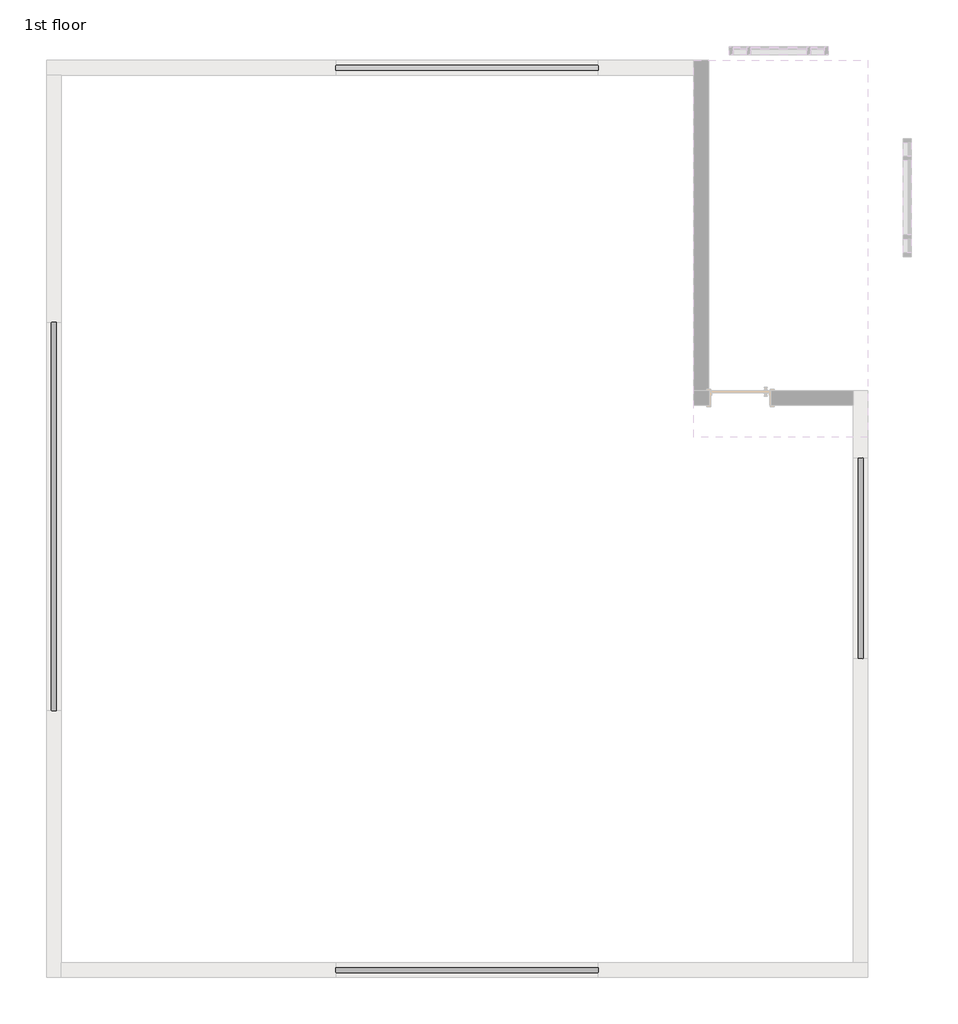
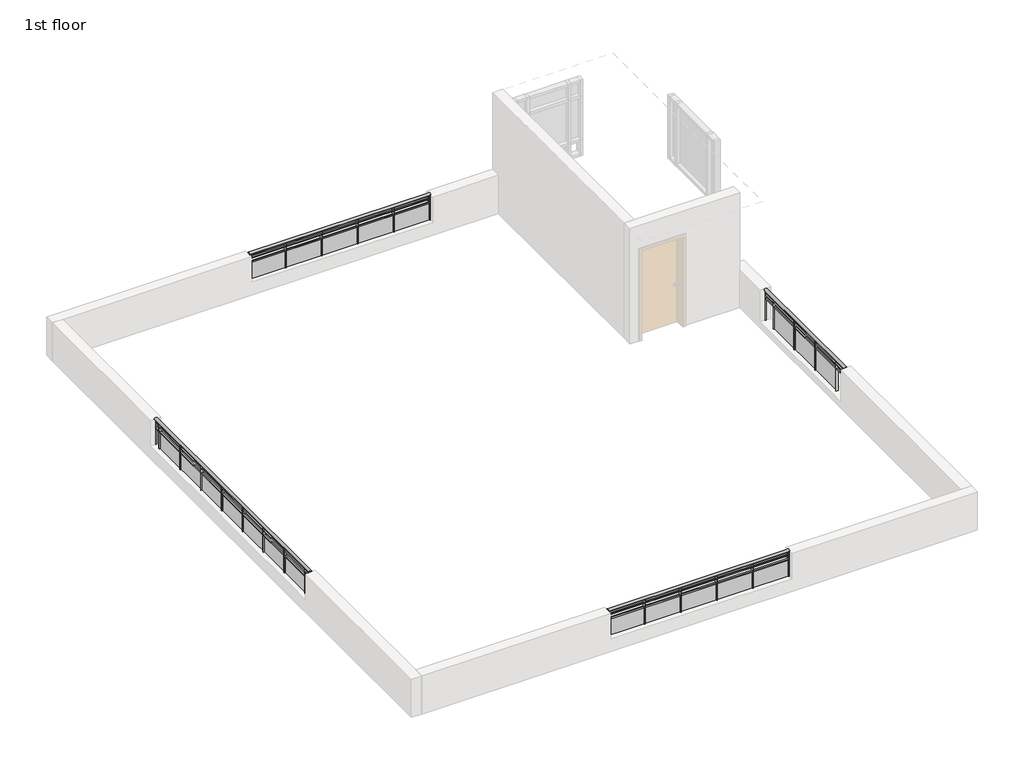
# One storey, part 2 of 2: 4 railings.
"""IFC4 building model written with IfcOpenShell, lengths in millimetres."""

from ifc_helpers import new_model, si_unit, point, frame, origin, place, context, project, spatial, polyline, ellipse_curve, trimmed, outline, extrude, element, save
from ifc_brep_helpers import plane_surface, extruded_surface, advanced_brep

model = new_model("IFC4")

# Units and contexts
model_context = context("Model", 3, world=origin())
ifc_project = project(units=[si_unit("LENGTHUNIT", "METRE", prefix="MILLI")], contexts=[model_context])

# Site, building, storey
site = spatial("IfcSite", under=ifc_project)
building = spatial("IfcBuilding", under=site)
storey = spatial("IfcBuildingStorey", under=building, Name="1st floor", Elevation=3200.4)

# Railings
placement = place(None, origin())
element("IfcRailing", 1, ObjectType="Glass Panel - Bottom Fill", at=placement, inside=storey, context=model_context, shape_type="SolidModel", body=[
    advanced_brep(
    [(186.9722402, 5808.6342801, 4086.225), (110.7722402, 5808.6342801, 4086.225), (186.9722402, 2680.2485536, 4086.225), (110.7722402, 2680.2485536, 4086.225)],
    [
        (0, 1, ellipse_curve(frame((148.8722402, 5808.6342801, 4086.225), z_axis=(0.0, 1.0, 0.0), x_axis=(-1.0, 0.0, 0.0)), 38.1, 28.575)),
        (1, 0, ellipse_curve(frame((148.8722402, 5808.6342801, 4086.225), z_axis=(0.0, 1.0, 0.0), x_axis=(-1.0, 0.0, 0.0)), 38.1, 28.575)),
        (2, 3, ellipse_curve(frame((148.8722402, 2680.2485536, 4086.225), z_axis=(0.0, -1.0, 0.0), x_axis=(-1.0, 0.0, 0.0)), 38.1, 28.575)),
        (3, 2, ellipse_curve(frame((148.8722402, 2680.2485536, 4086.225), z_axis=(0.0, -1.0, 0.0), x_axis=(-1.0, 0.0, 0.0)), 38.1, 28.575)),
        (0, 2),
        (3, 1),
    ],
    [
        plane_surface(frame((148.8722402, 5808.6342801, 4086.225), z_axis=(0.0, 1.0, 0.0), x_axis=(0.0, 0.0, -1.0))),
        plane_surface(frame((148.8722402, 2680.2485536, 4086.225), z_axis=(0.0, -1.0, 0.0), x_axis=(0.0, 0.0, -1.0))),
        extruded_surface(trimmed(ellipse_curve(frame((148.8722402, 2680.2485536, 4086.225), z_axis=(0.0, 1.0, 0.0), x_axis=(-1.0, 0.0, 0.0)), 38.1, 28.575), [point((186.9722402, 2680.2485536, 4086.225))], [point((110.7722402, 2680.2485536, 4086.225))], True, "CARTESIAN"), (0.0, 3128.3857265, 0.0), 3128.3857265),
        extruded_surface(trimmed(ellipse_curve(frame((148.8722402, 2680.2485536, 4086.225), z_axis=(0.0, 1.0, 0.0), x_axis=(-1.0, 0.0, 0.0)), 38.1, 28.575), [point((110.7722402, 2680.2485536, 4086.225))], [point((186.9722402, 2680.2485536, 4086.225))], True, "CARTESIAN"), (0.0, 3128.3857265, 0.0), 3128.3857265),
    ],
    [
        (0, [[1, 2]]),
        (1, [[3, 4]]),
        (2, [[-1, 5, -4, 6]]),
        (3, [[-2, -6, -3, -5]]),
    ],
),
    extrude(outline(polyline([(136.1722402, 5808.6342801), (161.5722402, 5808.6342801), (161.5722402, 2680.2485536), (136.1722402, 2680.2485536), (136.1722402, 5808.6342801)])), frame((0.0, 0.0, 3971.925), z_axis=(0.0, 0.0, 1.0), x_axis=(1.0, 0.0, 0.0)), (0.0, 0.0, 1.0), 25.4),
    extrude(outline(polyline([(136.1722402, 5808.6342801), (161.5722402, 5808.6342801), (161.5722402, 2680.2485536), (136.1722402, 2680.2485536), (136.1722402, 5808.6342801)])), frame((0.0, 0.0, 3870.325), z_axis=(0.0, 0.0, 1.0), x_axis=(1.0, 0.0, 0.0)), (0.0, 0.0, 1.0), 25.4),
    extrude(outline(polyline([(123.4722402, 3031.5914169), (174.2722402, 3031.5914169), (174.2722402, 3018.8914169), (123.4722402, 3018.8914169), (123.4722402, 3031.5914169)])), frame((0.0, 0.0, 3171.825), z_axis=(0.0, 0.0, 1.0), x_axis=(1.0, 0.0, 0.0)), (0.0, 0.0, 1.0), 885.825),
    extrude(outline(polyline([(155.4073972, 3838.0414169), (155.4073972, 3025.2414169), (149.0573972, 3025.2414169), (149.0573972, 3838.0414169), (155.4073972, 3838.0414169)])), frame((0.0, 0.0, 3273.425), z_axis=(0.0, 0.0, 1.0), x_axis=(1.0, 0.0, 0.0)), (0.0, 0.0, 1.0), 596.9),
    extrude(outline(polyline([(123.4722402, 3844.3914169), (174.2722402, 3844.3914169), (174.2722402, 3831.6914169), (123.4722402, 3831.6914169), (123.4722402, 3844.3914169)])), frame((0.0, 0.0, 3171.825), z_axis=(0.0, 0.0, 1.0), x_axis=(1.0, 0.0, 0.0)), (0.0, 0.0, 1.0), 885.825),
    extrude(outline(polyline([(155.4073972, 4650.8414169), (155.4073972, 3838.0414169), (149.0573972, 3838.0414169), (149.0573972, 4650.8414169), (155.4073972, 4650.8414169)])), frame((0.0, 0.0, 3273.425), z_axis=(0.0, 0.0, 1.0), x_axis=(1.0, 0.0, 0.0)), (0.0, 0.0, 1.0), 596.9),
    extrude(outline(polyline([(123.4722402, 4657.1914169), (174.2722402, 4657.1914169), (174.2722402, 4644.4914169), (123.4722402, 4644.4914169), (123.4722402, 4657.1914169)])), frame((0.0, 0.0, 3171.825), z_axis=(0.0, 0.0, 1.0), x_axis=(1.0, 0.0, 0.0)), (0.0, 0.0, 1.0), 885.825),
    extrude(outline(polyline([(155.4073972, 5463.6414169), (155.4073972, 4650.8414169), (149.0573972, 4650.8414169), (149.0573972, 5463.6414169), (155.4073972, 5463.6414169)])), frame((0.0, 0.0, 3273.425), z_axis=(0.0, 0.0, 1.0), x_axis=(1.0, 0.0, 0.0)), (0.0, 0.0, 1.0), 596.9),
    extrude(outline(polyline([(123.4722402, 5469.9914169), (174.2722402, 5469.9914169), (174.2722402, 5457.2914169), (123.4722402, 5457.2914169), (123.4722402, 5469.9914169)])), frame((0.0, 0.0, 3171.825), z_axis=(0.0, 0.0, 1.0), x_axis=(1.0, 0.0, 0.0)), (0.0, 0.0, 1.0), 885.825),
    extrude(outline(polyline([(139.3472402, 2692.9485536), (158.3972402, 2692.9485536), (158.3972402, 2673.8985536), (139.3472402, 2673.8985536), (139.3472402, 2692.9485536)])), frame((0.0, 0.0, 3171.825), z_axis=(0.0, 0.0, 1.0), x_axis=(1.0, 0.0, 0.0)), (0.0, 0.0, 1.0), 885.825),
    extrude(outline(polyline([(139.3472402, 5814.9842801), (158.3972402, 5814.9842801), (158.3972402, 5795.9342801), (139.3472402, 5795.9342801), (139.3472402, 5814.9842801)])), frame((0.0, 0.0, 3171.825), z_axis=(0.0, 0.0, 1.0), x_axis=(1.0, 0.0, 0.0)), (0.0, 0.0, 1.0), 885.825),
])
element("IfcRailing", 2, ObjectType="Glass Panel - Bottom Fill", at=placement, inside=storey, context=model_context, shape_type="SolidModel", body=[
    advanced_brep(
    [(-8005.6015325, -2116.1657199, 4114.8), (-8005.6015325, -2192.3657199, 4114.8), (-3926.753987, -2116.1657199, 4114.8), (-3926.753987, -2192.3657199, 4114.8)],
    [
        (0, 1, ellipse_curve(frame((-8005.6015325, -2154.2657199, 4114.8), z_axis=(-1.0, 0.0, 0.0), x_axis=(0.0, -1.0, 0.0)), 38.1, 28.575)),
        (1, 0, ellipse_curve(frame((-8005.6015325, -2154.2657199, 4114.8), z_axis=(-1.0, 0.0, 0.0), x_axis=(0.0, -1.0, 0.0)), 38.1, 28.575)),
        (2, 3, ellipse_curve(frame((-3926.753987, -2154.2657199, 4114.8), z_axis=(1.0, 0.0, 0.0), x_axis=(0.0, -1.0, 0.0)), 38.1, 28.575)),
        (3, 2, ellipse_curve(frame((-3926.753987, -2154.2657199, 4114.8), z_axis=(1.0, 0.0, 0.0), x_axis=(0.0, -1.0, 0.0)), 38.1, 28.575)),
        (0, 2),
        (3, 1),
    ],
    [
        plane_surface(frame((-8005.6015325, -2154.2657199, 4114.8), z_axis=(-1.0, 0.0, 0.0), x_axis=(0.0, 1.0, 0.0))),
        plane_surface(frame((-3926.753987, -2154.2657199, 4114.8), z_axis=(1.0, 0.0, 0.0), x_axis=(0.0, 1.0, 0.0))),
        extruded_surface(trimmed(ellipse_curve(frame((-3926.753987, -2154.2657199, 4114.8), z_axis=(-1.0, 0.0, 0.0), x_axis=(0.0, -1.0, 0.0)), 38.1, 28.575), [point((-3926.753987, -2116.1657199, 4114.8))], [point((-3926.753987, -2192.3657199, 4114.8))], True, "CARTESIAN"), (-4078.8475455, 0.0, 0.0), 4078.8475455),
        extruded_surface(trimmed(ellipse_curve(frame((-3926.753987, -2154.2657199, 4114.8), z_axis=(-1.0, 0.0, 0.0), x_axis=(0.0, -1.0, 0.0)), 38.1, 28.575), [point((-3926.753987, -2192.3657199, 4114.8))], [point((-3926.753987, -2116.1657199, 4114.8))], True, "CARTESIAN"), (-4078.8475455, 0.0, 0.0), 4078.8475455),
    ],
    [
        (0, [[1, 2]]),
        (1, [[3, 4]]),
        (2, [[-1, 5, -4, 6]]),
        (3, [[-2, -6, -3, -5]]),
    ],
),
    extrude(outline(polyline([(-8005.6015325, -2166.9657199), (-8005.6015325, -2141.5657199), (-3926.753987, -2141.5657199), (-3926.753987, -2166.9657199), (-8005.6015325, -2166.9657199)])), frame((0.0, 0.0, 4000.5), z_axis=(0.0, 0.0, 1.0), x_axis=(1.0, 0.0, 0.0)), (0.0, 0.0, 1.0), 25.4),
    extrude(outline(polyline([(-8005.6015325, -2166.9657199), (-8005.6015325, -2141.5657199), (-3926.753987, -2141.5657199), (-3926.753987, -2166.9657199), (-8005.6015325, -2166.9657199)])), frame((0.0, 0.0, 3898.9), z_axis=(0.0, 0.0, 1.0), x_axis=(1.0, 0.0, 0.0)), (0.0, 0.0, 1.0), 25.4),
    extrude(outline(polyline([(-3940.5277598, -2179.6657199), (-3940.5277598, -2128.8657199), (-3927.8277598, -2128.8657199), (-3927.8277598, -2179.6657199), (-3940.5277598, -2179.6657199)])), frame((0.0, 0.0, 3200.4), z_axis=(0.0, 0.0, 1.0), x_axis=(1.0, 0.0, 0.0)), (0.0, 0.0, 1.0), 885.825),
    extrude(outline(polyline([(-4746.9777598, -2147.7305629), (-3934.1777598, -2147.7305629), (-3934.1777598, -2154.0805629), (-4746.9777598, -2154.0805629), (-4746.9777598, -2147.7305629)])), frame((0.0, 0.0, 3302.0), z_axis=(0.0, 0.0, 1.0), x_axis=(1.0, 0.0, 0.0)), (0.0, 0.0, 1.0), 596.9),
    extrude(outline(polyline([(-4753.3277598, -2179.6657199), (-4753.3277598, -2128.8657199), (-4740.6277598, -2128.8657199), (-4740.6277598, -2179.6657199), (-4753.3277598, -2179.6657199)])), frame((0.0, 0.0, 3200.4), z_axis=(0.0, 0.0, 1.0), x_axis=(1.0, 0.0, 0.0)), (0.0, 0.0, 1.0), 885.825),
    extrude(outline(polyline([(-5559.7777598, -2147.7305629), (-4746.9777598, -2147.7305629), (-4746.9777598, -2154.0805629), (-5559.7777598, -2154.0805629), (-5559.7777598, -2147.7305629)])), frame((0.0, 0.0, 3302.0), z_axis=(0.0, 0.0, 1.0), x_axis=(1.0, 0.0, 0.0)), (0.0, 0.0, 1.0), 596.9),
    extrude(outline(polyline([(-5566.1277598, -2179.6657199), (-5566.1277598, -2128.8657199), (-5553.4277598, -2128.8657199), (-5553.4277598, -2179.6657199), (-5566.1277598, -2179.6657199)])), frame((0.0, 0.0, 3200.4), z_axis=(0.0, 0.0, 1.0), x_axis=(1.0, 0.0, 0.0)), (0.0, 0.0, 1.0), 885.825),
    extrude(outline(polyline([(-6372.5777598, -2147.7305629), (-5559.7777598, -2147.7305629), (-5559.7777598, -2154.0805629), (-6372.5777598, -2154.0805629), (-6372.5777598, -2147.7305629)])), frame((0.0, 0.0, 3302.0), z_axis=(0.0, 0.0, 1.0), x_axis=(1.0, 0.0, 0.0)), (0.0, 0.0, 1.0), 596.9),
    extrude(outline(polyline([(-6378.9277598, -2179.6657199), (-6378.9277598, -2128.8657199), (-6366.2277598, -2128.8657199), (-6366.2277598, -2179.6657199), (-6378.9277598, -2179.6657199)])), frame((0.0, 0.0, 3200.4), z_axis=(0.0, 0.0, 1.0), x_axis=(1.0, 0.0, 0.0)), (0.0, 0.0, 1.0), 885.825),
    extrude(outline(polyline([(-7185.3777598, -2147.7305629), (-6372.5777598, -2147.7305629), (-6372.5777598, -2154.0805629), (-7185.3777598, -2154.0805629), (-7185.3777598, -2147.7305629)])), frame((0.0, 0.0, 3302.0), z_axis=(0.0, 0.0, 1.0), x_axis=(1.0, 0.0, 0.0)), (0.0, 0.0, 1.0), 596.9),
    extrude(outline(polyline([(-7191.7277598, -2179.6657199), (-7191.7277598, -2128.8657199), (-7179.0277598, -2128.8657199), (-7179.0277598, -2179.6657199), (-7191.7277598, -2179.6657199)])), frame((0.0, 0.0, 3200.4), z_axis=(0.0, 0.0, 1.0), x_axis=(1.0, 0.0, 0.0)), (0.0, 0.0, 1.0), 885.825),
    extrude(outline(polyline([(-7998.1777598, -2147.7305629), (-7185.3777598, -2147.7305629), (-7185.3777598, -2154.0805629), (-7998.1777598, -2154.0805629), (-7998.1777598, -2147.7305629)])), frame((0.0, 0.0, 3302.0), z_axis=(0.0, 0.0, 1.0), x_axis=(1.0, 0.0, 0.0)), (0.0, 0.0, 1.0), 596.9),
    extrude(outline(polyline([(-8004.5277598, -2179.6657199), (-8004.5277598, -2128.8657199), (-7991.8277598, -2128.8657199), (-7991.8277598, -2179.6657199), (-8004.5277598, -2179.6657199)])), frame((0.0, 0.0, 3200.4), z_axis=(0.0, 0.0, 1.0), x_axis=(1.0, 0.0, 0.0)), (0.0, 0.0, 1.0), 885.825),
    extrude(outline(polyline([(-3939.453987, -2163.7907199), (-3939.453987, -2144.7407199), (-3920.403987, -2144.7407199), (-3920.403987, -2163.7907199), (-3939.453987, -2163.7907199)])), frame((0.0, 0.0, 3200.4), z_axis=(0.0, 0.0, 1.0), x_axis=(1.0, 0.0, 0.0)), (0.0, 0.0, 1.0), 885.825),
    extrude(outline(polyline([(-8011.9515325, -2163.7907199), (-8011.9515325, -2144.7407199), (-7992.9015325, -2144.7407199), (-7992.9015325, -2163.7907199), (-8011.9515325, -2163.7907199)])), frame((0.0, 0.0, 3200.4), z_axis=(0.0, 0.0, 1.0), x_axis=(1.0, 0.0, 0.0)), (0.0, 0.0, 1.0), 885.825),
])
element("IfcRailing", 3, ObjectType="Glass Panel - Bottom Fill", at=placement, inside=storey, context=model_context, shape_type="SolidModel", body=[
    advanced_brep(
    [(-12347.9277598, 7909.3467978, 4114.8), (-12424.1277598, 7909.3467978, 4114.8), (-12347.9277598, 1879.1217625, 4114.8), (-12424.1277598, 1879.1217625, 4114.8)],
    [
        (0, 1, ellipse_curve(frame((-12386.0277598, 7909.3467978, 4114.8), z_axis=(0.0, 1.0, 0.0), x_axis=(-1.0, 0.0, 0.0)), 38.1, 28.575)),
        (1, 0, ellipse_curve(frame((-12386.0277598, 7909.3467978, 4114.8), z_axis=(0.0, 1.0, 0.0), x_axis=(-1.0, 0.0, 0.0)), 38.1, 28.575)),
        (2, 3, ellipse_curve(frame((-12386.0277598, 1879.1217625, 4114.8), z_axis=(0.0, -1.0, 0.0), x_axis=(-1.0, 0.0, 0.0)), 38.1, 28.575)),
        (3, 2, ellipse_curve(frame((-12386.0277598, 1879.1217625, 4114.8), z_axis=(0.0, -1.0, 0.0), x_axis=(-1.0, 0.0, 0.0)), 38.1, 28.575)),
        (0, 2),
        (3, 1),
    ],
    [
        plane_surface(frame((-12386.0277598, 7909.3467978, 4114.8), z_axis=(0.0, 1.0, 0.0), x_axis=(0.0, 0.0, -1.0))),
        plane_surface(frame((-12386.0277598, 1879.1217625, 4114.8), z_axis=(0.0, -1.0, 0.0), x_axis=(0.0, 0.0, -1.0))),
        extruded_surface(trimmed(ellipse_curve(frame((-12386.0277598, 1879.1217625, 4114.8), z_axis=(0.0, 1.0, 0.0), x_axis=(-1.0, 0.0, 0.0)), 38.1, 28.575), [point((-12347.9277598, 1879.1217625, 4114.8))], [point((-12424.1277598, 1879.1217625, 4114.8))], True, "CARTESIAN"), (0.0, 6030.2250353, 0.0), 6030.2250353),
        extruded_surface(trimmed(ellipse_curve(frame((-12386.0277598, 1879.1217625, 4114.8), z_axis=(0.0, 1.0, 0.0), x_axis=(-1.0, 0.0, 0.0)), 38.1, 28.575), [point((-12424.1277598, 1879.1217625, 4114.8))], [point((-12347.9277598, 1879.1217625, 4114.8))], True, "CARTESIAN"), (0.0, 6030.2250353, 0.0), 6030.2250353),
    ],
    [
        (0, [[1, 2]]),
        (1, [[3, 4]]),
        (2, [[-1, 5, -4, 6]]),
        (3, [[-2, -6, -3, -5]]),
    ],
),
    extrude(outline(polyline([(-12398.7277598, 7909.3467978), (-12373.3277598, 7909.3467978), (-12373.3277598, 1879.1217625), (-12398.7277598, 1879.1217625), (-12398.7277598, 7909.3467978)])), frame((0.0, 0.0, 4000.5), z_axis=(0.0, 0.0, 1.0), x_axis=(1.0, 0.0, 0.0)), (0.0, 0.0, 1.0), 25.4),
    extrude(outline(polyline([(-12398.7277598, 7909.3467978), (-12373.3277598, 7909.3467978), (-12373.3277598, 1879.1217625), (-12398.7277598, 1879.1217625), (-12398.7277598, 7909.3467978)])), frame((0.0, 0.0, 3898.9), z_axis=(0.0, 0.0, 1.0), x_axis=(1.0, 0.0, 0.0)), (0.0, 0.0, 1.0), 25.4),
    extrude(outline(polyline([(-12411.4277598, 2055.7842801), (-12360.6277598, 2055.7842801), (-12360.6277598, 2043.0842801), (-12411.4277598, 2043.0842801), (-12411.4277598, 2055.7842801)])), frame((0.0, 0.0, 3200.4), z_axis=(0.0, 0.0, 1.0), x_axis=(1.0, 0.0, 0.0)), (0.0, 0.0, 1.0), 885.825),
    extrude(outline(polyline([(-12379.4926028, 2862.2342801), (-12379.4926028, 2049.4342801), (-12385.8426028, 2049.4342801), (-12385.8426028, 2862.2342801), (-12379.4926028, 2862.2342801)])), frame((0.0, 0.0, 3302.0), z_axis=(0.0, 0.0, 1.0), x_axis=(1.0, 0.0, 0.0)), (0.0, 0.0, 1.0), 596.9),
    extrude(outline(polyline([(-12411.4277598, 2868.5842801), (-12360.6277598, 2868.5842801), (-12360.6277598, 2855.8842801), (-12411.4277598, 2855.8842801), (-12411.4277598, 2868.5842801)])), frame((0.0, 0.0, 3200.4), z_axis=(0.0, 0.0, 1.0), x_axis=(1.0, 0.0, 0.0)), (0.0, 0.0, 1.0), 885.825),
    extrude(outline(polyline([(-12379.4926028, 3675.0342801), (-12379.4926028, 2862.2342801), (-12385.8426028, 2862.2342801), (-12385.8426028, 3675.0342801), (-12379.4926028, 3675.0342801)])), frame((0.0, 0.0, 3302.0), z_axis=(0.0, 0.0, 1.0), x_axis=(1.0, 0.0, 0.0)), (0.0, 0.0, 1.0), 596.9),
    extrude(outline(polyline([(-12411.4277598, 3681.3842801), (-12360.6277598, 3681.3842801), (-12360.6277598, 3668.6842801), (-12411.4277598, 3668.6842801), (-12411.4277598, 3681.3842801)])), frame((0.0, 0.0, 3200.4), z_axis=(0.0, 0.0, 1.0), x_axis=(1.0, 0.0, 0.0)), (0.0, 0.0, 1.0), 885.825),
    extrude(outline(polyline([(-12379.4926028, 4487.8342801), (-12379.4926028, 3675.0342801), (-12385.8426028, 3675.0342801), (-12385.8426028, 4487.8342801), (-12379.4926028, 4487.8342801)])), frame((0.0, 0.0, 3302.0), z_axis=(0.0, 0.0, 1.0), x_axis=(1.0, 0.0, 0.0)), (0.0, 0.0, 1.0), 596.9),
    extrude(outline(polyline([(-12411.4277598, 4494.1842801), (-12360.6277598, 4494.1842801), (-12360.6277598, 4481.4842801), (-12411.4277598, 4481.4842801), (-12411.4277598, 4494.1842801)])), frame((0.0, 0.0, 3200.4), z_axis=(0.0, 0.0, 1.0), x_axis=(1.0, 0.0, 0.0)), (0.0, 0.0, 1.0), 885.825),
    extrude(outline(polyline([(-12379.4926028, 5300.6342801), (-12379.4926028, 4487.8342801), (-12385.8426028, 4487.8342801), (-12385.8426028, 5300.6342801), (-12379.4926028, 5300.6342801)])), frame((0.0, 0.0, 3302.0), z_axis=(0.0, 0.0, 1.0), x_axis=(1.0, 0.0, 0.0)), (0.0, 0.0, 1.0), 596.9),
    extrude(outline(polyline([(-12411.4277598, 5306.9842801), (-12360.6277598, 5306.9842801), (-12360.6277598, 5294.2842801), (-12411.4277598, 5294.2842801), (-12411.4277598, 5306.9842801)])), frame((0.0, 0.0, 3200.4), z_axis=(0.0, 0.0, 1.0), x_axis=(1.0, 0.0, 0.0)), (0.0, 0.0, 1.0), 885.825),
    extrude(outline(polyline([(-12379.4926028, 6113.4342801), (-12379.4926028, 5300.6342801), (-12385.8426028, 5300.6342801), (-12385.8426028, 6113.4342801), (-12379.4926028, 6113.4342801)])), frame((0.0, 0.0, 3302.0), z_axis=(0.0, 0.0, 1.0), x_axis=(1.0, 0.0, 0.0)), (0.0, 0.0, 1.0), 596.9),
    extrude(outline(polyline([(-12411.4277598, 6119.7842801), (-12360.6277598, 6119.7842801), (-12360.6277598, 6107.0842801), (-12411.4277598, 6107.0842801), (-12411.4277598, 6119.7842801)])), frame((0.0, 0.0, 3200.4), z_axis=(0.0, 0.0, 1.0), x_axis=(1.0, 0.0, 0.0)), (0.0, 0.0, 1.0), 885.825),
    extrude(outline(polyline([(-12379.4926028, 6926.2342801), (-12379.4926028, 6113.4342801), (-12385.8426028, 6113.4342801), (-12385.8426028, 6926.2342801), (-12379.4926028, 6926.2342801)])), frame((0.0, 0.0, 3302.0), z_axis=(0.0, 0.0, 1.0), x_axis=(1.0, 0.0, 0.0)), (0.0, 0.0, 1.0), 596.9),
    extrude(outline(polyline([(-12411.4277598, 6932.5842801), (-12360.6277598, 6932.5842801), (-12360.6277598, 6919.8842801), (-12411.4277598, 6919.8842801), (-12411.4277598, 6932.5842801)])), frame((0.0, 0.0, 3200.4), z_axis=(0.0, 0.0, 1.0), x_axis=(1.0, 0.0, 0.0)), (0.0, 0.0, 1.0), 885.825),
    extrude(outline(polyline([(-12379.4926028, 7739.0342801), (-12379.4926028, 6926.2342801), (-12385.8426028, 6926.2342801), (-12385.8426028, 7739.0342801), (-12379.4926028, 7739.0342801)])), frame((0.0, 0.0, 3302.0), z_axis=(0.0, 0.0, 1.0), x_axis=(1.0, 0.0, 0.0)), (0.0, 0.0, 1.0), 596.9),
    extrude(outline(polyline([(-12411.4277598, 7745.3842801), (-12360.6277598, 7745.3842801), (-12360.6277598, 7732.6842801), (-12411.4277598, 7732.6842801), (-12411.4277598, 7745.3842801)])), frame((0.0, 0.0, 3200.4), z_axis=(0.0, 0.0, 1.0), x_axis=(1.0, 0.0, 0.0)), (0.0, 0.0, 1.0), 885.825),
    extrude(outline(polyline([(-12395.5527598, 1891.8217625), (-12376.5027598, 1891.8217625), (-12376.5027598, 1872.7717625), (-12395.5527598, 1872.7717625), (-12395.5527598, 1891.8217625)])), frame((0.0, 0.0, 3200.4), z_axis=(0.0, 0.0, 1.0), x_axis=(1.0, 0.0, 0.0)), (0.0, 0.0, 1.0), 885.825),
    extrude(outline(polyline([(-12395.5527598, 7915.6967978), (-12376.5027598, 7915.6967978), (-12376.5027598, 7896.6467978), (-12395.5527598, 7896.6467978), (-12395.5527598, 7915.6967978)])), frame((0.0, 0.0, 3200.4), z_axis=(0.0, 0.0, 1.0), x_axis=(1.0, 0.0, 0.0)), (0.0, 0.0, 1.0), 885.825),
])
element("IfcRailing", 4, ObjectType="Glass Panel - Bottom Fill", at=placement, inside=storey, context=model_context, shape_type="SolidModel", body=[
    advanced_brep(
    [(-3926.753987, 11828.4342801, 4114.8), (-3926.753987, 11904.6342801, 4114.8), (-8005.6015325, 11828.4342801, 4114.8), (-8005.6015325, 11904.6342801, 4114.8)],
    [
        (0, 1, ellipse_curve(frame((-3926.753987, 11866.5342801, 4114.8), z_axis=(1.0, 0.0, 0.0), x_axis=(0.0, 1.0, 0.0)), 38.1, 28.575)),
        (1, 0, ellipse_curve(frame((-3926.753987, 11866.5342801, 4114.8), z_axis=(1.0, 0.0, 0.0), x_axis=(0.0, 1.0, 0.0)), 38.1, 28.575)),
        (2, 3, ellipse_curve(frame((-8005.6015325, 11866.5342801, 4114.8), z_axis=(-1.0, 0.0, 0.0), x_axis=(0.0, 1.0, 0.0)), 38.1, 28.575)),
        (3, 2, ellipse_curve(frame((-8005.6015325, 11866.5342801, 4114.8), z_axis=(-1.0, 0.0, 0.0), x_axis=(0.0, 1.0, 0.0)), 38.1, 28.575)),
        (0, 2),
        (3, 1),
    ],
    [
        plane_surface(frame((-3926.753987, 11866.5342801, 4114.8), z_axis=(1.0, 0.0, 0.0), x_axis=(0.0, -1.0, 0.0))),
        plane_surface(frame((-8005.6015325, 11866.5342801, 4114.8), z_axis=(-1.0, 0.0, 0.0), x_axis=(0.0, -1.0, 0.0))),
        extruded_surface(trimmed(ellipse_curve(frame((-8005.6015325, 11866.5342801, 4114.8), z_axis=(1.0, 0.0, 0.0), x_axis=(0.0, 1.0, 0.0)), 38.1, 28.575), [point((-8005.6015325, 11828.4342801, 4114.8))], [point((-8005.6015325, 11904.6342801, 4114.8))], True, "CARTESIAN"), (4078.8475455, 0.0, 0.0), 4078.8475455),
        extruded_surface(trimmed(ellipse_curve(frame((-8005.6015325, 11866.5342801, 4114.8), z_axis=(1.0, 0.0, 0.0), x_axis=(0.0, 1.0, 0.0)), 38.1, 28.575), [point((-8005.6015325, 11904.6342801, 4114.8))], [point((-8005.6015325, 11828.4342801, 4114.8))], True, "CARTESIAN"), (4078.8475455, 0.0, 0.0), 4078.8475455),
    ],
    [
        (0, [[1, 2]]),
        (1, [[3, 4]]),
        (2, [[-1, 5, -4, 6]]),
        (3, [[-2, -6, -3, -5]]),
    ],
),
    extrude(outline(polyline([(-3926.753987, 11879.2342801), (-3926.753987, 11853.8342801), (-8005.6015325, 11853.8342801), (-8005.6015325, 11879.2342801), (-3926.753987, 11879.2342801)])), frame((0.0, 0.0, 4000.5), z_axis=(0.0, 0.0, 1.0), x_axis=(1.0, 0.0, 0.0)), (0.0, 0.0, 1.0), 25.4),
    extrude(outline(polyline([(-3926.753987, 11879.2342801), (-3926.753987, 11853.8342801), (-8005.6015325, 11853.8342801), (-8005.6015325, 11879.2342801), (-3926.753987, 11879.2342801)])), frame((0.0, 0.0, 3898.9), z_axis=(0.0, 0.0, 1.0), x_axis=(1.0, 0.0, 0.0)), (0.0, 0.0, 1.0), 25.4),
    extrude(outline(polyline([(-7991.8277598, 11891.9342801), (-7991.8277598, 11841.1342801), (-8004.5277598, 11841.1342801), (-8004.5277598, 11891.9342801), (-7991.8277598, 11891.9342801)])), frame((0.0, 0.0, 3200.4), z_axis=(0.0, 0.0, 1.0), x_axis=(1.0, 0.0, 0.0)), (0.0, 0.0, 1.0), 885.825),
    extrude(outline(polyline([(-7185.3777598, 11859.9991231), (-7998.1777598, 11859.9991231), (-7998.1777598, 11866.3491231), (-7185.3777598, 11866.3491231), (-7185.3777598, 11859.9991231)])), frame((0.0, 0.0, 3302.0), z_axis=(0.0, 0.0, 1.0), x_axis=(1.0, 0.0, 0.0)), (0.0, 0.0, 1.0), 596.9),
    extrude(outline(polyline([(-7179.0277598, 11891.9342801), (-7179.0277598, 11841.1342801), (-7191.7277598, 11841.1342801), (-7191.7277598, 11891.9342801), (-7179.0277598, 11891.9342801)])), frame((0.0, 0.0, 3200.4), z_axis=(0.0, 0.0, 1.0), x_axis=(1.0, 0.0, 0.0)), (0.0, 0.0, 1.0), 885.825),
    extrude(outline(polyline([(-6372.5777598, 11859.9991231), (-7185.3777598, 11859.9991231), (-7185.3777598, 11866.3491231), (-6372.5777598, 11866.3491231), (-6372.5777598, 11859.9991231)])), frame((0.0, 0.0, 3302.0), z_axis=(0.0, 0.0, 1.0), x_axis=(1.0, 0.0, 0.0)), (0.0, 0.0, 1.0), 596.9),
    extrude(outline(polyline([(-6366.2277598, 11891.9342801), (-6366.2277598, 11841.1342801), (-6378.9277598, 11841.1342801), (-6378.9277598, 11891.9342801), (-6366.2277598, 11891.9342801)])), frame((0.0, 0.0, 3200.4), z_axis=(0.0, 0.0, 1.0), x_axis=(1.0, 0.0, 0.0)), (0.0, 0.0, 1.0), 885.825),
    extrude(outline(polyline([(-5559.7777598, 11859.9991231), (-6372.5777598, 11859.9991231), (-6372.5777598, 11866.3491231), (-5559.7777598, 11866.3491231), (-5559.7777598, 11859.9991231)])), frame((0.0, 0.0, 3302.0), z_axis=(0.0, 0.0, 1.0), x_axis=(1.0, 0.0, 0.0)), (0.0, 0.0, 1.0), 596.9),
    extrude(outline(polyline([(-5553.4277598, 11891.9342801), (-5553.4277598, 11841.1342801), (-5566.1277598, 11841.1342801), (-5566.1277598, 11891.9342801), (-5553.4277598, 11891.9342801)])), frame((0.0, 0.0, 3200.4), z_axis=(0.0, 0.0, 1.0), x_axis=(1.0, 0.0, 0.0)), (0.0, 0.0, 1.0), 885.825),
    extrude(outline(polyline([(-4746.9777598, 11859.9991231), (-5559.7777598, 11859.9991231), (-5559.7777598, 11866.3491231), (-4746.9777598, 11866.3491231), (-4746.9777598, 11859.9991231)])), frame((0.0, 0.0, 3302.0), z_axis=(0.0, 0.0, 1.0), x_axis=(1.0, 0.0, 0.0)), (0.0, 0.0, 1.0), 596.9),
    extrude(outline(polyline([(-4740.6277598, 11891.9342801), (-4740.6277598, 11841.1342801), (-4753.3277598, 11841.1342801), (-4753.3277598, 11891.9342801), (-4740.6277598, 11891.9342801)])), frame((0.0, 0.0, 3200.4), z_axis=(0.0, 0.0, 1.0), x_axis=(1.0, 0.0, 0.0)), (0.0, 0.0, 1.0), 885.825),
    extrude(outline(polyline([(-3934.1777598, 11859.9991231), (-4746.9777598, 11859.9991231), (-4746.9777598, 11866.3491231), (-3934.1777598, 11866.3491231), (-3934.1777598, 11859.9991231)])), frame((0.0, 0.0, 3302.0), z_axis=(0.0, 0.0, 1.0), x_axis=(1.0, 0.0, 0.0)), (0.0, 0.0, 1.0), 596.9),
    extrude(outline(polyline([(-3927.8277598, 11891.9342801), (-3927.8277598, 11841.1342801), (-3940.5277598, 11841.1342801), (-3940.5277598, 11891.9342801), (-3927.8277598, 11891.9342801)])), frame((0.0, 0.0, 3200.4), z_axis=(0.0, 0.0, 1.0), x_axis=(1.0, 0.0, 0.0)), (0.0, 0.0, 1.0), 885.825),
    extrude(outline(polyline([(-7992.9015325, 11876.0592801), (-7992.9015325, 11857.0092801), (-8011.9515325, 11857.0092801), (-8011.9515325, 11876.0592801), (-7992.9015325, 11876.0592801)])), frame((0.0, 0.0, 3200.4), z_axis=(0.0, 0.0, 1.0), x_axis=(1.0, 0.0, 0.0)), (0.0, 0.0, 1.0), 885.825),
    extrude(outline(polyline([(-3920.403987, 11876.0592801), (-3920.403987, 11857.0092801), (-3939.453987, 11857.0092801), (-3939.453987, 11876.0592801), (-3920.403987, 11876.0592801)])), frame((0.0, 0.0, 3200.4), z_axis=(0.0, 0.0, 1.0), x_axis=(1.0, 0.0, 0.0)), (0.0, 0.0, 1.0), 885.825),
])

save(model, "model.ifc")

# Revit data of these elements
# Type "Glass Panel - Bottom Fill"
#   built-in parameter 1008612 = 0.0416667 (stored number, unit not read)
#   built-in parameter 1008611 = 0.0416667 (stored number, unit not read)
#   built-in parameter 1008609 = 0.333333 (stored number, unit not read)
#   built-in parameter 1008604 = 0.166667 (stored number, unit not read)
#   built-in parameter 1008603 = 0.166667 (stored number, unit not read)
#   Railing Height = 3' - 0"
#   built-in parameter 1008630 = 2
#   built-in parameter 1008610 = 2
#   built-in parameter 1008618 = Baluster - Square : 3/4"
# Element 1 (IfcRailing, "Glass Panel - Bottom Fill")
#   built-in parameter 1008621 = -0.09375 (stored number, unit not read)
#   Phase Created = New Construction
#   Materials on its faces: "Glass"
# Elements 2, 3, 4 (IfcRailing, "Glass Panel - Bottom Fill")
#   Phase Created = New Construction
#   Materials on its faces: "Glass"
# Materials
#   "Glass": class "Glass", colour RGB 0 128 192, transparency 0.75, Description = "Soda Lime Glass", Cost = 0
